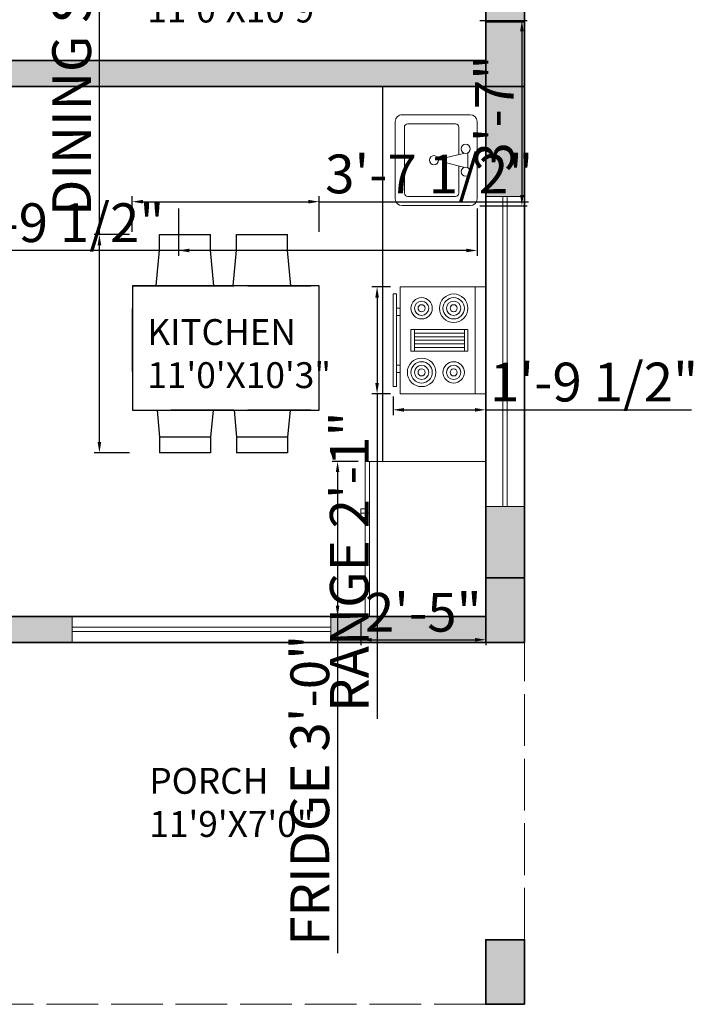
# Model space of a CAD drawing. Units: inches. Extents: x 3148 to 3962, y 1142 to 1671.
# Tile 2 of 9: x 3365 to 3521, y 1198 to 1426. Entities that reach past the tile are written whole.
import ezdxf

# ---------------------------------------------------------------- set-up
doc = ezdxf.new("R2010")
doc.units = ezdxf.units.IN
doc.linetypes.add('ACAD_ISO02W100', pattern=[15, 12, -3])
for name, color, linetype, lineweight in [('A-ANNO-DIMS', 2, 'Continuous', 18), ('A-AREA-IDEN', 7, 'Continuous', 18), ('A-COLS', 1, 'Continuous', 35), ('A-EQPM', 9, 'Continuous', 18), ('A-FLOR-CASE', 8, 'Continuous', 25), ('A-FLOR-FIXT', 21, 'Continuous', 18), ('A-FURN', 8, 'Continuous', 18), ('A-GLAZ', 4, 'Continuous', 18), ('A-ROOF-OVHD', 7, 'ACAD_ISO02W100', 18), ('A-WALL', 7, 'Continuous', 35)]:
    doc.layers.add(name, color=color, linetype=linetype, lineweight=lineweight)
doc.layers.add('A-WALL-PATT', color=252, linetype='Continuous', lineweight=13, true_color=0x939598)
doc.layers.add('NOI THAT', color=42, linetype='Continuous')
doc.styles.add('ATT', font='romans.shx')
doc.styles.get("Standard").update_dxf_attribs({"font": 'arial.ttf'})
doc.dimstyles.new('ISO-25', dxfattribs={"dimtxt": 9, "dimasz": 2.5, "dimexe": 1.25, "dimexo": 0.625, "dimtad": 1, "dimdec": 1, "dimlunit": 3, "dimtxsty": 'Standard', "dimcen": 2.5, "dimadec": 0, "dimazin": 0, "dimtfac": 1, "dimtdec": 1, "dimtmove": 0, "dimatfit": 3, "dimfxl": 1, "dimarcsym": 0})

# ---------------------------------------------------------------- blocks, each defined once
blk = doc.blocks.new('A$C755A44B5')
at = {"layer": 'NOI THAT'}
for p, q in [((176.7, 1403.2), (503.6, 1403.2)), ((176.7, 1303.2), (176.7, 1403.2)), ((503.6, 1303.2), (503.6, 1403.2)), ((671.9, 1403.2), (998.8, 1403.2)), ((671.9, 1303.2), (671.9, 1403.2)), ((998.8, 1303.2), (998.8, 1403.2)), ((154.6, 1073.7), (176.7, 1303.2)), ((176.7, 1303.2), (503.6, 1303.2)), ((525.7, 1073.7), (503.6, 1303.2)), ((649.8, 1073.7), (671.9, 1303.2)), ((671.9, 1303.2), (998.8, 1303.2)), ((1020.9, 1073.7), (998.8, 1303.2)), ((2, 1073.7), (2, 273.7)), ((1202, 1073.7), (2, 1073.7)), ((2, 1073.7), (452, 1073.7)), ((2, 1073.7), (2, 723.7)), ((249.5, 1073.7), (654.5, 1073.7)), ((744.7, 1073.7), (1149.7, 1073.7)), ((1202, 273.7), (1202, 1073.7)), ((0, 927), (0, 522)), ((2, 273.7), (1202, 273.7)), ((160, 273.7), (176.7, 100)), ((654.5, 273.7), (249.5, 273.7)), ((520.3, 273.7), (503.6, 100)), ((655.2, 273.7), (671.9, 100)), ((1149.7, 273.7), (744.7, 273.7)), ((1015.5, 273.7), (998.8, 100)), ((503.6, 100), (176.7, 100)), ((176.7, 100), (176.7, 0)), ((503.6, 100), (503.6, 0)), ((998.8, 100), (671.9, 100)), ((671.9, 100), (671.9, 0)), ((998.8, 100), (998.8, 0)), ((503.6, 0), (176.7, 0)), ((998.8, 0), (671.9, 0))]:
    blk.add_line(p, q, dxfattribs=at)
blk = doc.blocks.new('Refrigerator-2 door - 36 in top')
for p, q in [((0, -26.999999), (36, -26.999999)), ((12, -26.999999), (12, -28.999999)), ((11, -27.999999), (11, -28.999999)), ((11, -28.999999), (13, -28.999999)), ((13, -28.999999), (13, -27.999999))]:
    blk.add_line(p, q)
blk.add_lwpolyline([(0, -27.999999), (0, 0), (36, 0), (36, -27.999999)], close=True)
blk = doc.blocks.new('Range-Oven - 30 in top')
for p, q in [((0, -3), (30, -3)), ((12, -6), (18, -6)), ((13, -20), (13, -6)), ((14, -6), (14, -20)), ((15, -20), (15, -6)), ((16, -6), (16, -20)), ((17, -20), (17, -6)), ((18, -20), (12, -20)), ((6, -24), (6, -25)), ((8, -25), (8, -24)), ((22, -25), (22, -24)), ((24, -24), (24, -25))]:
    blk.add_line(p, q)
for points in [[(0, -24), (0, 0), (30, 0), (30, -24)], [(12, -21), (12, -5), (18, -5), (18, -21)], [(2, -26), (2, -25), (28, -25), (28, -26)]]:
    blk.add_lwpolyline(points, close=True)
for centre, radius in [((6, -9), 4), ((6, -9), 3), ((6, -9), 2), ((6, -9), 1), ((24, -9), 3), ((24, -9), 2), ((24, -9), 1), ((6, -18), 3), ((6, -18), 2), ((24, -18), 4), ((24, -18), 3), ((24, -18), 2), ((6, -18), 1), ((24, -18), 1)]:
    blk.add_circle(centre, radius)
blk = doc.blocks.new('15PLAV06')
at = {"color": 0, "linetype": 'ByBlock'}
for p, q in [((16.5, 10), (1.5, 10)), ((0, 8.5), (0, -8.5)), ((4, 1.25), (4, 7.25)), ((4.75, 8), (15.25, 8)), ((16, 7.25), (16, -7.25)), ((18, -8.5), (18, 8.5)), ((2, -1.5), (2, 1.5)), ((7, 0.5), (3, 1.5)), ((7, -0.5), (7, 0.5)), ((3, -1.5), (7, -0.5)), ((4, -7.25), (4, -1.25)), ((15.25, -8), (4.75, -8)), ((1.5, -10), (16.5, -10))]:
    blk.add_line(p, q, dxfattribs=at)
for centre in [(2.5, 2.5), (9.5, 0), (2.5, -2.5)]:
    blk.add_circle(centre, 1, dxfattribs=at)
for centre, radius, start, end in [((1.5, 8.5), 1.5, 90, 180), ((16.5, 8.5), 1.5, 0, 90), ((4.75, 7.25), 0.75, 90, 180), ((15.25, 7.25), 0.75, 0, 90), ((1.5, -8.5), 1.5, 180, 270), ((4.75, -7.25), 0.75, 180, 270), ((15.25, -7.25), 0.75, 270, 0), ((16.5, -8.5), 1.5, 270, 0)]:
    blk.add_arc(centre, radius, start, end, dxfattribs=at)
at = {"color": 0, "linetype": 'ByBlock', "style": 'ATT'}
for tag, p, flags in [('ITEM', (0, -20), 3), ('ROOM_NUMBER', (0, -29), 1)]:
    blk.add_attdef(tag, p, '', height=6, dxfattribs=dict(at, flags=flags))
blk = doc.blocks.new('WIN-60')
for p, q in [((0, 0), (0, 6)), ((60, 0), (60, 6)), ((60, 3.5), (0, 3.5)), ((60, 2.5), (0, 2.5))]:
    blk.add_line(p, q)
blk = doc.blocks.new('WIN-72')
for p, q in [((0, 72), (9, 72)), ((4, 72), (4, 0)), ((5, 72), (5, 0)), ((0, 0), (9, 0))]:
    blk.add_line(p, q)
blk = doc.blocks.new('COL-9X15')
h = blk.add_hatch(color=256)
h.dxf.hatch_style = 1
h.paths.add_polyline_path([(9, 15), (0, 15), (0, 0), (9, 0)])
blk.add_lwpolyline([(9, 0), (9, 15), (0, 15), (0, 0)], close=True)
blk = doc.blocks.new('*D94')
at = {"layer": 'A-ANNO-DIMS', "color": 0, "lineweight": -2, "transparency": 16777216}
for p, q in [((3379.97, 1444.32), (3379.97, 1429.73)), ((3473.04, 1444.32), (3473.04, 1429.73)), ((3382.47, 1430.98), (3470.54, 1430.98))]:
    blk.add_line(p, q, dxfattribs=at)
at = {"layer": 'A-ANNO-DIMS', "color": 0, "transparency": 16777216}
for points in [[(3382.47, 1431.4), (3382.47, 1430.57), (3379.97, 1430.98)], [(3470.54, 1431.4), (3470.54, 1430.57), (3473.04, 1430.98)]]:
    blk.add_solid(points, dxfattribs=at)
at = {"layer": 'Defpoints', "color": 0, "transparency": 16777216}
for p in [(3379.97, 1444.95), (3473.04, 1444.95), (3473.04, 1430.98)]:
    blk.add_point(p, dxfattribs=at)
at = {"layer": 'A-ANNO-DIMS', "color": 0, "transparency": 16777216, "insert": (3426.51, 1436.2), "char_height": 9, "attachment_point": 5}
blk.add_mtext('BED 7\'-9"', dxfattribs=at)
blk = doc.blocks.new('*D96')
at = {"layer": 'A-ANNO-DIMS', "color": 0, "lineweight": -2, "transparency": 16777216}
for p, q in [((3383.35, 1376.46), (3383.35, 1500.1)), ((3390.32, 1376.46), (3382.1, 1376.46)), ((3383.35, 1328.3), (3383.35, 1373.96)), ((3390.32, 1325.8), (3382.1, 1325.8))]:
    blk.add_line(p, q, dxfattribs=at)
at = {"layer": 'A-ANNO-DIMS', "color": 0, "transparency": 16777216}
for points in [[(3382.93, 1373.96), (3383.77, 1373.96), (3383.35, 1376.46)], [(3382.93, 1328.3), (3383.77, 1328.3), (3383.35, 1325.8)]]:
    blk.add_solid(points, dxfattribs=at)
at = {"layer": 'Defpoints', "color": 0, "transparency": 16777216}
for p in [(3383.35, 1376.46), (3390.95, 1376.46), (3390.95, 1325.8)]:
    blk.add_point(p, dxfattribs=at)
at = {"layer": 'A-ANNO-DIMS', "color": 0, "transparency": 16777216, "insert": (3378.07, 1439.53), "char_height": 9, "attachment_point": 5, "rotation": 90}
blk.add_mtext('DINING SET 4\'-2 1/2"', dxfattribs=at)
blk = doc.blocks.new('*D97')
at = {"layer": 'A-ANNO-DIMS', "color": 0, "lineweight": -2, "transparency": 16777216}
for p, q in [((3390.95, 1377.09), (3390.95, 1385.31)), ((3434.34, 1377.09), (3434.34, 1385.31)), ((3393.45, 1384.06), (3431.84, 1384.06)), ((3434.34, 1384.06), (3482.98, 1384.06))]:
    blk.add_line(p, q, dxfattribs=at)
at = {"layer": 'A-ANNO-DIMS', "color": 0, "transparency": 16777216}
for points in [[(3393.45, 1384.48), (3393.45, 1383.64), (3390.95, 1384.06)], [(3431.84, 1384.48), (3431.84, 1383.64), (3434.34, 1384.06)]]:
    blk.add_solid(points, dxfattribs=at)
at = {"layer": 'Defpoints', "color": 0, "transparency": 16777216}
for p in [(3434.34, 1384.06), (3390.95, 1376.46), (3434.34, 1376.46)]:
    blk.add_point(p, dxfattribs=at)
at = {"layer": 'A-ANNO-DIMS', "color": 0, "transparency": 16777216, "insert": (3459.91, 1389.34), "char_height": 9, "attachment_point": 5}
blk.add_mtext('3\'-7 1/2"', dxfattribs=at)
blk = doc.blocks.new('*D104')
at = {"layer": 'A-ANNO-DIMS', "color": 0, "lineweight": -2, "transparency": 16777216}
for p, q in [((3443.42, 1323.8), (3437.39, 1323.8)), ((3438.64, 1321.3), (3438.64, 1290.3)), ((3443.42, 1287.8), (3437.39, 1287.8)), ((3438.64, 1287.8), (3438.64, 1209.64))]:
    blk.add_line(p, q, dxfattribs=at)
at = {"layer": 'A-ANNO-DIMS', "color": 0, "transparency": 16777216}
for points in [[(3438.23, 1321.3), (3439.06, 1321.3), (3438.64, 1323.8)], [(3438.23, 1290.3), (3439.06, 1290.3), (3438.64, 1287.8)]]:
    blk.add_solid(points, dxfattribs=at)
at = {"layer": 'Defpoints', "color": 0, "transparency": 16777216}
for p in [(3444.04, 1323.8), (3438.64, 1287.8), (3444.04, 1287.8)]:
    blk.add_point(p, dxfattribs=at)
at = {"layer": 'A-ANNO-DIMS', "color": 0, "transparency": 16777216, "insert": (3433.36, 1247.47), "char_height": 9, "attachment_point": 5, "rotation": 90}
blk.add_mtext('FRIDGE 3\'-0"', dxfattribs=at)
blk = doc.blocks.new('*D105')
at = {"layer": 'A-ANNO-DIMS', "color": 0, "lineweight": -2, "transparency": 16777216}
for p, q in [((3444.04, 1287.17), (3444.04, 1281.15)), ((3473.04, 1287.17), (3473.04, 1281.15)), ((3446.54, 1282.4), (3470.54, 1282.4))]:
    blk.add_line(p, q, dxfattribs=at)
at = {"layer": 'A-ANNO-DIMS', "color": 0, "transparency": 16777216}
for points in [[(3446.54, 1282.82), (3446.54, 1281.98), (3444.04, 1282.4)], [(3470.54, 1282.82), (3470.54, 1281.98), (3473.04, 1282.4)]]:
    blk.add_solid(points, dxfattribs=at)
at = {"layer": 'Defpoints', "color": 0, "transparency": 16777216}
for p in [(3444.04, 1287.8), (3473.04, 1287.8), (3473.04, 1282.4)]:
    blk.add_point(p, dxfattribs=at)
at = {"layer": 'A-ANNO-DIMS', "color": 0, "transparency": 16777216, "insert": (3458.54, 1287.62), "char_height": 9, "attachment_point": 5}
blk.add_mtext('2\'-5"', dxfattribs=at)
blk = doc.blocks.new('*D106')
at = {"layer": 'A-ANNO-DIMS', "color": 0, "lineweight": -2, "transparency": 16777216}
for p, q in [((3450.91, 1364.3), (3446.56, 1364.3)), ((3447.81, 1361.8), (3447.81, 1341.98)), ((3450.91, 1339.48), (3446.56, 1339.48)), ((3447.81, 1339.48), (3447.81, 1264.07))]:
    blk.add_line(p, q, dxfattribs=at)
at = {"layer": 'A-ANNO-DIMS', "color": 0, "transparency": 16777216}
for points in [[(3447.39, 1361.8), (3448.23, 1361.8), (3447.81, 1364.3)], [(3447.39, 1341.98), (3448.23, 1341.98), (3447.81, 1339.48)]]:
    blk.add_solid(points, dxfattribs=at)
at = {"layer": 'Defpoints', "color": 0, "transparency": 16777216}
for p in [(3451.53, 1364.3), (3447.81, 1339.48), (3451.53, 1339.48)]:
    blk.add_point(p, dxfattribs=at)
at = {"layer": 'A-ANNO-DIMS', "color": 0, "transparency": 16777216, "insert": (3442.53, 1300.52), "char_height": 9, "attachment_point": 5, "rotation": 90}
blk.add_mtext('RANGE 2\'-1"', dxfattribs=at)
blk = doc.blocks.new('*D107')
at = {"layer": 'A-ANNO-DIMS', "color": 0, "lineweight": -2, "transparency": 16777216}
for p, q in [((3451.53, 1338.86), (3451.53, 1334.51)), ((3473.04, 1338.86), (3473.04, 1334.51)), ((3454.03, 1335.76), (3470.54, 1335.76)), ((3473.04, 1335.76), (3520.84, 1335.76))]:
    blk.add_line(p, q, dxfattribs=at)
at = {"layer": 'A-ANNO-DIMS', "color": 0, "transparency": 16777216}
for points in [[(3454.03, 1336.17), (3454.03, 1335.34), (3451.53, 1335.76)], [(3470.54, 1336.17), (3470.54, 1335.34), (3473.04, 1335.76)]]:
    blk.add_solid(points, dxfattribs=at)
at = {"layer": 'Defpoints', "color": 0, "transparency": 16777216}
for p in [(3451.53, 1339.48), (3473.04, 1339.48), (3473.04, 1335.76)]:
    blk.add_point(p, dxfattribs=at)
at = {"layer": 'A-ANNO-DIMS', "color": 0, "transparency": 16777216, "insert": (3498.19, 1341.04), "char_height": 9, "attachment_point": 5}
blk.add_mtext('1\'-9 1/2"', dxfattribs=at)
blk = doc.blocks.new('*D108')
at = {"layer": 'A-ANNO-DIMS', "color": 0, "lineweight": -2, "transparency": 16777216}
for p, q in [((3401.7, 1382.52), (3401.7, 1371.49)), ((3471.03, 1382.52), (3471.03, 1371.49)), ((3401.7, 1372.74), (3287.44, 1372.74)), ((3468.53, 1372.74), (3404.2, 1372.74))]:
    blk.add_line(p, q, dxfattribs=at)
at = {"layer": 'A-ANNO-DIMS', "color": 0, "transparency": 16777216}
for points in [[(3404.2, 1373.16), (3404.2, 1372.33), (3401.7, 1372.74)], [(3468.53, 1373.16), (3468.53, 1372.33), (3471.03, 1372.74)]]:
    blk.add_solid(points, dxfattribs=at)
at = {"layer": 'Defpoints', "color": 0, "transparency": 16777216}
for p in [(3401.7, 1383.14), (3471.03, 1383.14), (3401.7, 1372.74)]:
    blk.add_point(p, dxfattribs=at)
at = {"layer": 'A-ANNO-DIMS', "color": 0, "transparency": 16777216, "insert": (3343.32, 1378.02), "char_height": 9, "attachment_point": 5}
blk.add_mtext('SINK UNIT 5\'-9 1/2"', dxfattribs=at)
blk = doc.blocks.new('*D109')
at = {"layer": 'A-ANNO-DIMS', "color": 0, "lineweight": -2, "transparency": 16777216}
for p, q in [((3471.66, 1426.08), (3482.68, 1426.08)), ((3481.43, 1423.58), (3481.43, 1385.64)), ((3471.66, 1383.14), (3482.68, 1383.14))]:
    blk.add_line(p, q, dxfattribs=at)
at = {"layer": 'A-ANNO-DIMS', "color": 0, "transparency": 16777216}
for points in [[(3481.02, 1423.58), (3481.85, 1423.58), (3481.43, 1426.08)], [(3481.02, 1385.64), (3481.85, 1385.64), (3481.43, 1383.14)]]:
    blk.add_solid(points, dxfattribs=at)
at = {"layer": 'Defpoints', "color": 0, "transparency": 16777216}
for p in [(3471.03, 1426.08), (3471.03, 1383.14), (3481.43, 1383.14)]:
    blk.add_point(p, dxfattribs=at)
at = {"layer": 'A-ANNO-DIMS', "color": 0, "transparency": 16777216, "insert": (3476.21, 1404.61), "char_height": 9, "attachment_point": 5, "rotation": 90}
blk.add_mtext('3\'-7"', dxfattribs=at)

msp = doc.modelspace()

# ---------------------------------------------------------------- hatches: boundary and pattern name
at = {"layer": 'A-WALL-PATT'}
h = msp.add_hatch(color=256, dxfattribs=at)
h.dxf.hatch_style = 1
h.paths.add_polyline_path([(3203.04, 1410.8), (3194.04, 1410.8), (3194.04, 1296.8), (3203.04, 1296.8), (3203.04, 1300.86)])
h.paths.add_polyline_path([(3203.04, 1281.8), (3194.04, 1281.8), (3194.04, 1212.8), (3203.04, 1212.8)])
h.paths.add_polyline_path([(3326.04, 1206.8), (3203.04, 1206.8), (3203.04, 1197.8), (3326.04, 1197.8)])
h.paths.add_polyline_path([(3341.04, 1362.8), (3335.04, 1362.8), (3335.04, 1290.8), (3341.04, 1290.8)])
h.paths.add_polyline_path([(3341.04, 1207.8), (3335.04, 1207.8), (3335.04, 1206.8), (3341.04, 1206.8)])
h.paths.add_polyline_path([(3341.04, 1259.8), (3335.04, 1259.8), (3335.04, 1255.8), (3341.04, 1255.8)])
h.paths.add_polyline_path([(3341.04, 1281.8), (3335.04, 1281.8), (3335.04, 1277.8), (3341.04, 1277.8)])
h.paths.add_polyline_path([(3377.04, 1287.8), (3350.04, 1287.8), (3350.04, 1281.8), (3377.04, 1281.8)])
h.paths.add_polyline_path([(3473.04, 1287.8), (3445.04, 1287.8), (3437.04, 1287.8), (3437.04, 1281.8), (3473.04, 1281.8)])
h.paths.add_polyline_path([(3482.04, 1313.3), (3473.04, 1313.3), (3473.04, 1296.8), (3482.04, 1296.8)])
h.paths.add_polyline_path([(3482.04, 1410.8), (3473.04, 1410.8), (3473.04, 1385.3), (3482.04, 1385.3)])
h.paths.add_polyline_path([(3473.04, 1416.8), (3344.04, 1416.8), (3344.04, 1410.8), (3473.04, 1410.8)])
h.paths.add_polyline_path([(3482.04, 1445.3), (3473.04, 1445.3), (3473.04, 1425.8), (3482.04, 1425.8)])
h.paths.add_polyline_path([(3341.04, 1426.3), (3335.04, 1426.3), (3335.04, 1425.8), (3341.04, 1425.8)])
h.paths.add_polyline_path([(3304.04, 1428.8), (3253.54, 1428.8), (3253.54, 1430.3), (3251.04, 1430.3), (3251.04, 1428.8), (3203.04, 1428.8), (3203.04, 1512.8), (3215.04, 1512.8), (3215.04, 1518.8), (3203.04, 1518.8), (3203.04, 1539.8), (3194.04, 1539.8), (3194.04, 1425.8), (3203.04, 1425.8), (3203.04, 1422.8), (3304.04, 1422.8)])
h.paths.add_polyline_path([(3265.54, 1518.8), (3239.04, 1518.8), (3239.04, 1512.8), (3251.04, 1512.8), (3251.04, 1461.3), (3253.54, 1461.3), (3253.54, 1462.3), (3255.54, 1462.3), (3255.54, 1464.8), (3253.54, 1464.8), (3253.54, 1512.8), (3265.54, 1512.8)], flags=17)
h.paths.add_polyline_path([(3307.54, 1518.8), (3289.54, 1518.8), (3289.54, 1512.8), (3301.54, 1512.8), (3301.54, 1464.8), (3286.54, 1464.8), (3286.54, 1462.3), (3304.04, 1462.3), (3304.04, 1512.8), (3307.54, 1512.8)])
h.paths.add_polyline_path([(3341.04, 1539.8), (3335.04, 1539.8), (3335.04, 1518.8), (3331.54, 1518.8), (3331.54, 1512.8), (3335.04, 1512.8), (3335.04, 1462.3), (3341.04, 1462.3)])
h.paths.add_polyline_path([(3335.04, 1554.8), (3203.04, 1554.8), (3203.04, 1545.8), (3335.04, 1545.8)])
h.paths.add_polyline_path([(3473.04, 1554.8), (3344.04, 1554.8), (3344.04, 1545.8), (3362.94, 1545.8), (3473.04, 1545.8)])
h.paths.add_polyline_path([(3482.04, 1539.8), (3473.04, 1539.8), (3473.04, 1517.3), (3482.04, 1517.3)])

# ---------------------------------------------------------------- linework, layer by layer
at = {"layer": 'A-FLOR-CASE'}
msp.add_line((3449.04, 1410.8), (3449.04, 1323.8), dxfattribs=at)
at = {"layer": 'A-ROOF-OVHD'}
for p, q in [((3482.04, 1197.8), (3482.04, 1281.8)), ((3341.04, 1197.8), (3482.04, 1197.8))]:
    msp.add_line(p, q, dxfattribs=at)
at = {"layer": 'A-WALL'}
for p, q in [((3482.04, 1554.8), (3482.04, 1281.8)), ((3473.04, 1545.8), (3473.04, 1416.8)), ((3473.04, 1416.8), (3341.04, 1416.8)), ((3473.04, 1410.8), (3335.04, 1410.8)), ((3473.04, 1410.8), (3473.04, 1287.8)), ((3341.04, 1287.8), (3473.04, 1287.8)), ((3341.04, 1281.8), (3473.04, 1281.8))]:
    msp.add_line(p, q, dxfattribs=at)

# ---------------------------------------------------------------- block references
at = {"layer": 'A-COLS'}
for p in [(3473.04, 1410.8), (3473.04, 1281.8), (3473.04, 1197.8)]:
    msp.add_blockref('COL-9X15', p, dxfattribs=at)
at = {"layer": 'A-EQPM', "xscale": 0.8273016567796815, "yscale": 0.8273016567796815, "zscale": 0.8273016567796815, "rotation": 270}
msp.add_blockref('Range-Oven - 30 in top', (3473.04, 1364.3), dxfattribs=at)
at = {"layer": 'A-EQPM', "rotation": 270}
msp.add_blockref('Refrigerator-2 door - 36 in top', (3473.04, 1323.8), dxfattribs=at)
at = {"layer": 'A-FLOR-FIXT', "xscale": 1.054623354967256, "yscale": 1.054623354967256, "zscale": 1.054623354967256, "rotation": 180}
msp.add_blockref('15PLAV06', (3471.03, 1393.69), dxfattribs=at)
at = {"layer": 'A-FURN', "xscale": 0.0361004849165552, "yscale": 0.0361004849165552, "zscale": 0.0361004849165552}
msp.add_blockref('A$C755A44B5', (3390.95, 1325.8), dxfattribs=at)
at = {"layer": 'A-GLAZ'}
msp.add_blockref('WIN-72', (3473.04, 1313.3), dxfattribs=at)
at = {"layer": 'A-GLAZ', "rotation": 180}
msp.add_blockref('WIN-60', (3437.04, 1287.8), dxfattribs=at)

# ---------------------------------------------------------------- texts
at = {"layer": 'A-AREA-IDEN', "char_height": 6, "attachment_point": 1}
for s, insert in [('BEDROOM\\P11\'0\'X10\'9"', (3394.47, 1441.65)), ('KITCHEN\\P11\'0\'X10\'3"', (3394.47, 1356.81)), ('PORCH\\P11\'9\'X7\'0"', (3394.94, 1252.65))]:
    msp.add_mtext_dynamic_manual_height_columns(s, width=77.9518, gutter_width=12.5, heights=[0], dxfattribs=dict(at, insert=insert))

# ---------------------------------------------------------------- dimensions: what is measured, and where the dimension line sits
at = {"layer": 'A-ANNO-DIMS'}
for base, p1, p2, angle, text, picture, middle in [((3383.35, 1376.46), (3390.95, 1325.8), (3390.95, 1376.46), 90, 'DINING SET <>', '*D96', (3378.07, 1439.53)), ((3401.7, 1372.74), (3471.03, 1383.14), (3401.7, 1383.14), 180, 'SINK UNIT <>', '*D108', (3343.32, 1378.02)), ((3447.81, 1339.48), (3451.53, 1364.3), (3451.53, 1339.48), 270, 'RANGE <>', '*D106', (3442.53, 1300.52)), ((3438.64, 1287.8), (3444.04, 1323.8), (3444.04, 1287.8), 270, 'FRIDGE <>', '*D104', (3433.36, 1247.47))]:
    dim = msp.add_linear_dim(base=base, p1=p1, p2=p2, angle=angle, text=text, dimstyle='ISO-25', override={"dimdec": 1, "dimlfac": 1, "dimrnd": 0, "dimzin": 1, "dimdsep": 46, "dimlunit": 4, "dimfrac": 2}, dxfattribs=at)
    dim.commit()
    dim.dimension.update_dxf_attribs({"geometry": picture, "text_midpoint": middle})
dim = msp.add_linear_dim(base=(3473.04, 1430.98), p1=(3379.97, 1444.95), p2=(3473.04, 1444.95), text='BED <>', dimstyle='ISO-25', override={"dimdec": 1, "dimlfac": 1, "dimrnd": 0, "dimzin": 1, "dimdsep": 46, "dimlunit": 4, "dimfrac": 2}, dxfattribs=at)
dim.commit()
dim.dimension.update_dxf_attribs({"geometry": '*D94', "text_midpoint": (3426.51, 1436.2)})
dim = msp.add_linear_dim(base=(3481.43, 1383.14), p1=(3471.03, 1426.08), p2=(3471.03, 1383.14), angle=270, dimstyle='ISO-25', override={"dimdec": 1, "dimlfac": 1, "dimrnd": 0, "dimzin": 1, "dimdsep": 46, "dimlunit": 4, "dimfrac": 2}, dxfattribs=at)
dim.commit()
dim.dimension.update_dxf_attribs({"geometry": '*D109', "text_midpoint": (3476.21, 1404.61)})
for base, p1, p2, picture, middle in [((3434.34, 1384.06), (3390.95, 1376.46), (3434.34, 1376.46), '*D97', (3459.91, 1389.34)), ((3473.04, 1335.76), (3451.53, 1339.48), (3473.04, 1339.48), '*D107', (3498.19, 1341.04)), ((3473.04, 1282.4), (3444.04, 1287.8), (3473.04, 1287.8), '*D105', (3458.54, 1287.62))]:
    dim = msp.add_linear_dim(base=base, p1=p1, p2=p2, dimstyle='ISO-25', override={"dimdec": 1, "dimlfac": 1, "dimrnd": 0, "dimzin": 1, "dimdsep": 46, "dimlunit": 4, "dimfrac": 2}, dxfattribs=at)
    dim.commit()
    dim.dimension.update_dxf_attribs({"geometry": picture, "text_midpoint": middle})

doc.saveas('drawing.dxf')
